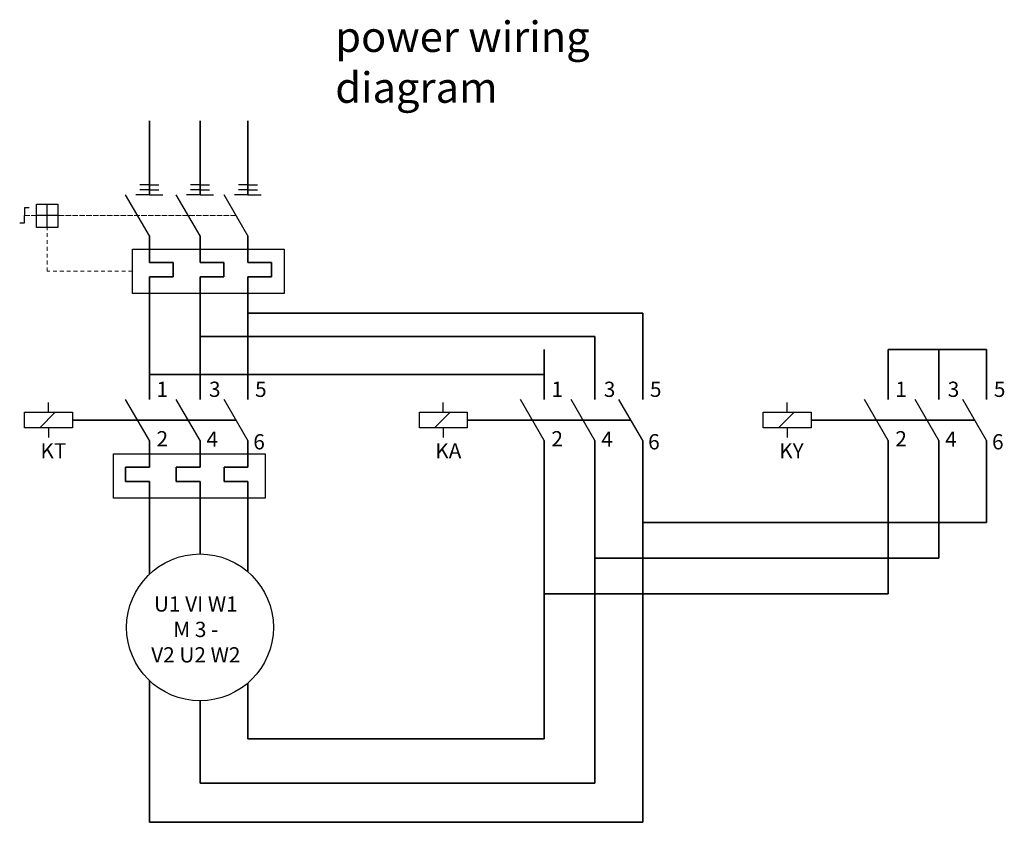
# Model space of a CAD drawing. Units: millimetres. Extents: x 37.3 to 69.6, y 11.5 to 37.8.
import ezdxf

# ---------------------------------------------------------------- set-up
doc = ezdxf.new("R2010")
doc.units = ezdxf.units.MM
doc.header["$MEASUREMENT"] = 0
doc.linetypes.add('HIDDEN2', pattern=[0.1875, 0.125, -0.0625])
for name, color, linetype, lineweight in [('E-ANNO-TEXT', 7, 'Continuous', 18), ('E-POWR-EQPM', 7, 'Continuous', 25), ('E-POWR-HIDN', 7, 'HIDDEN2', 18), ('E-POWR-WIRE', 1, 'Continuous', 35)]:
    doc.layers.add(name, color=color, linetype=linetype, lineweight=lineweight)
doc.styles.get("Standard").update_dxf_attribs({"font": 'arial.ttf'})

# ---------------------------------------------------------------- blocks, each defined once
blk = doc.blocks.new('CONTACTOR-3P')
for p, q in [((38.259, 24.888), (38.259, 25.209)), ((41.564, 23.958), (40.785, 25.307)), ((43.224, 23.958), (42.445, 25.307)), ((44.792, 23.958), (44.013, 25.307)), ((38.482, 24.888), (37.972, 24.377)), ((37.472, 24.633), (37.472, 24.633)), ((37.472, 24.633), (37.476, 24.633)), ((37.476, 24.633), (37.472, 24.633)), ((44.402, 24.633), (39.042, 24.633)), ((39.042, 24.633), (44.402, 24.633)), ((44.402, 24.633), (44.402, 24.633)), ((38.259, 24.377), (38.259, 24.057))]:
    blk.add_line(p, q)
blk.add_lwpolyline([(37.476, 24.888), (39.042, 24.888), (39.042, 24.377), (37.476, 24.377)], close=True)
blk = doc.blocks.new('BREAKER-POLE')
for p, q in [((41.564, 32.337), (41.252, 32.337)), ((41.564, 32.337), (41.875, 32.337)), ((41.564, 30.664), (40.785, 32.013)), ((41.564, 32.013), (41.123, 32.013)), ((41.564, 32.175), (41.252, 32.175)), ((41.564, 32.175), (41.875, 32.175)), ((41.564, 32.013), (42.005, 32.013))]:
    blk.add_line(p, q)

msp = doc.modelspace()

# ---------------------------------------------------------------- linework, layer by layer
at = {"layer": 'E-POWR-EQPM'}
for p, q in [((38.22, 30.937), (38.22, 31.708)), ((37.626, 31.583), (37.472, 31.583)), ((37.472, 31.583), (37.472, 31.338)), ((37.472, 31.093), (37.472, 31.338)), ((38.567, 31.338), (37.867, 31.338)), ((37.317, 31.093), (37.472, 31.093))]:
    msp.add_line(p, q, dxfattribs=at)
for points in [[(37.867, 31.708), (38.567, 31.708), (38.567, 30.937), (37.867, 30.937)], [(41.009, 30.229), (45.983, 30.229), (45.983, 28.782), (41.009, 28.782)], [(40.389, 23.523), (45.362, 23.523), (45.362, 22.077), (40.389, 22.077)]]:
    msp.add_lwpolyline(points, close=True, dxfattribs=at)
msp.add_circle((43.224, 17.838), 2.405, dxfattribs=at)
at = {"layer": 'E-POWR-HIDN'}
for p, q in [((38.22, 29.506), (38.22, 31.708)), ((41.009, 29.506), (38.22, 29.506))]:
    msp.add_line(p, q, dxfattribs=at)
msp.add_lwpolyline([(44.402, 31.338), (37.472, 31.338), (37.472, 31.338), (44.402, 31.338)], close=True, dxfattribs=at)
at = {"layer": 'E-POWR-WIRE'}
for p, q in [((41.564, 34.436), (41.564, 32.013)), ((43.224, 34.436), (43.224, 32.013)), ((44.792, 34.436), (44.792, 32.013)), ((41.564, 30.664), (41.564, 29.794)), ((43.224, 30.664), (43.224, 29.794)), ((44.792, 30.664), (44.792, 29.794)), ((41.564, 29.794), (42.341, 29.794)), ((42.341, 29.794), (42.341, 29.32)), ((43.224, 29.794), (44.001, 29.794)), ((44.001, 29.794), (44.001, 29.32)), ((44.792, 29.794), (45.569, 29.794)), ((45.569, 29.794), (45.569, 29.32)), ((42.341, 29.32), (41.564, 29.32)), ((41.564, 29.32), (41.564, 26.948)), ((43.224, 29.32), (43.224, 26.948)), ((44.001, 29.32), (43.224, 29.32)), ((44.792, 29.32), (44.792, 26.948)), ((45.569, 29.32), (44.792, 29.32)), ((44.792, 28.134), (57.726, 28.134)), ((57.726, 28.134), (57.726, 26.948)), ((43.224, 27.366), (56.158, 27.366)), ((56.158, 27.366), (56.158, 26.948)), ((41.564, 26.948), (41.564, 25.307)), ((43.224, 26.948), (43.224, 25.307)), ((44.792, 26.948), (44.792, 25.307)), ((54.498, 26.948), (54.498, 25.307)), ((56.158, 26.948), (56.158, 25.307)), ((57.726, 26.948), (57.726, 25.307)), ((65.765, 26.948), (65.765, 25.307)), ((65.765, 26.948), (68.993, 26.948)), ((67.425, 26.948), (67.425, 25.307)), ((68.993, 26.948), (68.993, 25.307)), ((41.564, 26.127), (54.498, 26.127)), ((41.564, 23.958), (41.564, 23.088)), ((43.224, 23.958), (43.224, 23.088)), ((44.792, 23.958), (44.792, 23.088)), ((54.498, 23.958), (54.498, 23.088)), ((56.158, 23.958), (56.158, 23.088)), ((57.726, 23.958), (57.726, 23.088)), ((65.765, 23.958), (65.765, 23.088)), ((67.425, 23.958), (67.425, 23.088)), ((68.993, 23.958), (68.993, 23.088)), ((41.564, 23.088), (40.786, 23.088)), ((40.786, 23.088), (40.786, 22.614)), ((43.224, 23.088), (42.446, 23.088)), ((42.446, 23.088), (42.446, 22.614)), ((44.792, 23.088), (44.014, 23.088)), ((44.014, 23.088), (44.014, 22.614)), ((54.498, 23.088), (54.498, 14.185)), ((56.158, 23.088), (56.158, 12.732)), ((57.726, 11.45), (57.726, 23.088)), ((65.765, 23.088), (65.765, 18.934)), ((67.425, 23.088), (67.425, 20.103)), ((68.993, 23.088), (68.993, 21.273)), ((40.786, 22.614), (41.564, 22.614)), ((41.564, 22.614), (41.564, 19.577)), ((42.446, 22.614), (43.224, 22.614)), ((43.224, 22.614), (43.224, 20.242)), ((44.014, 22.614), (44.792, 22.614)), ((44.792, 22.614), (44.792, 19.661)), ((68.993, 21.273), (57.726, 21.273)), ((67.425, 20.103), (56.158, 20.103)), ((65.765, 18.934), (54.498, 18.934)), ((41.564, 16.098), (41.564, 11.45)), ((44.792, 16.015), (44.792, 14.185)), ((43.224, 15.433), (43.224, 12.732)), ((54.498, 14.185), (44.792, 14.185)), ((56.158, 12.732), (43.224, 12.732)), ((41.564, 11.45), (52.487, 11.45)), ((52.487, 11.45), (57.726, 11.45))]:
    msp.add_line(p, q, dxfattribs=at)

# ---------------------------------------------------------------- block references
at = {"layer": 'E-POWR-EQPM'}
for name, p in [('BREAKER-POLE', (0, 0)), ('BREAKER-POLE', (1.66, 0)), ('BREAKER-POLE', (3.228, 0)), ('CONTACTOR-3P', (0, 0)), ('CONTACTOR-3P', (12.935, 0)), ('CONTACTOR-3P', (24.202, 0))]:
    msp.add_blockref(name, p, dxfattribs=at)

# ---------------------------------------------------------------- texts
at = {"layer": 'E-ANNO-TEXT', "attachment_point": 1}
for s, width, insert, char_height in [('{power wiring diagram}', 13.80755, (47.655, 37.694), 1), ('1', 1.36863, (41.801, 25.89), 0.5), ('3', 1.36863, (43.518, 25.89), 0.5), ('5', 1.36863, (45.028, 25.89), 0.5), ('1', 1.36863, (54.735, 25.89), 0.5), ('3', 1.36863, (56.452, 25.89), 0.5), ('5', 1.36863, (57.963, 25.89), 0.5), ('1', 1.36863, (66.002, 25.89), 0.5), ('3', 1.36863, (67.719, 25.89), 0.5), ('5', 1.36863, (69.23, 25.89), 0.5), ('2', 1.36863, (41.801, 24.269), 0.5), ('4', 1.36863, (43.435, 24.256), 0.5), ('2', 1.36863, (54.735, 24.269), 0.5), ('4', 1.36863, (56.369, 24.256), 0.5), ('2', 1.36863, (66.002, 24.269), 0.5), ('4', 1.36863, (67.636, 24.256), 0.5), ('KT', 1.36863, (37.997, 23.873), 0.5), ('6', 1.36863, (44.97, 24.17), 0.5), ('KA', 1.36863, (50.931, 23.873), 0.5), ('6', 1.36863, (57.904, 24.17), 0.5), ('KY', 1.36863, (62.198, 23.873), 0.5), ('6', 1.36863, (69.171, 24.17), 0.5), ('\\pxqc;U1 VI W1\\PM 3 -\\PV2 U2 W2', 3.77542, (41.199, 18.855), 0.5)]:
    msp.add_mtext_dynamic_manual_height_columns(s, width=width, gutter_width=1, heights=[0], dxfattribs=dict(at, insert=insert, char_height=char_height))

doc.saveas('drawing.dxf')
